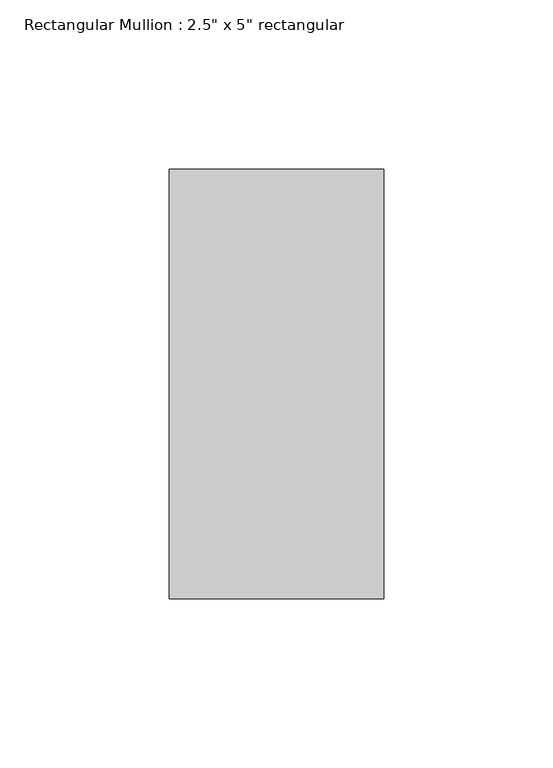
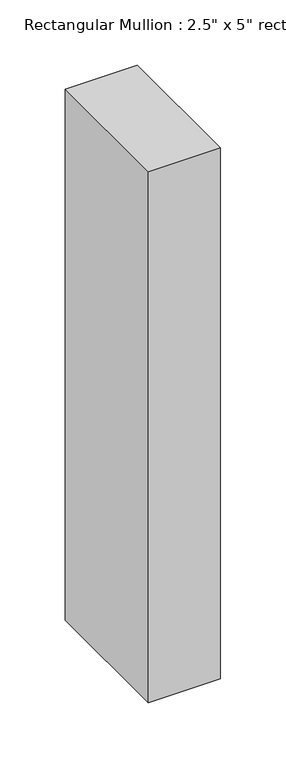
"""IFC4 building model written with IfcOpenShell, lengths in millimetres: member geometry."""

from ifc_helpers import new_model, si_unit, frame, origin, place, context, project, spatial, polyline, outline, extrude, source, transform, mapped, element, save


def member_9ab3e039(model_context):
    return source(origin(), model_context, "Body", "SweptSolid", [
        extrude(outline(polyline([(31.75, 63.5), (31.75, -63.5), (-31.75, -63.5), (-31.75, 63.5), (31.75, 63.5)])), frame((0.0, 0.0, -495.3), z_axis=(0.0, 0.0, 1.0), x_axis=(1.0, 0.0, 0.0)), (0.0, 0.0, 1.0), 495.3),
    ])


if __name__ == "__main__":
    model = new_model("IFC4")
    model_context = context("Model", 3, world=origin())
    ifc_project = project(units=[si_unit("LENGTHUNIT", "METRE", prefix="MILLI")], contexts=[model_context])
    site = spatial("IfcSite", under=ifc_project)
    building = spatial("IfcBuilding", under=site)
    placement = place(None, origin())
    member_shape = member_9ab3e039(model_context)
    element("IfcMember", 1, ObjectType="Rectangular Mullion : 2.5\" x 5\" rectangular", at=placement, inside=building, context=model_context, shape_type="MappedRepresentation", body=[
        mapped(member_shape, transform((0.0, 0.0, 0.0), x_axis=(1.0, 0.0, 0.0), y_axis=(0.0, 1.0, 0.0), z_axis=(0.0, 0.0, 1.0))),
    ])
    save(model, "model.ifc")

# Revit data of these elements
# Type "Rectangular Mullion : 2.5\" x 5\" rectangular"
#   built-in parameter 1007304 = 0.416667 (stored number, unit not read)
#   built-in parameter 1007301 = 0.104167 (stored number, unit not read)
#   built-in parameter 1007300 = 0.104167 (stored number, unit not read)
# Element 1 (IfcMember, "Rectangular Mullion : 2.5\" x 5\" rectangular")
#   Materials on its faces: "door colour"
# Materials
#   "door colour": class "Generic", colour RGB 120 120 120, transparency 0, Cost = 0
